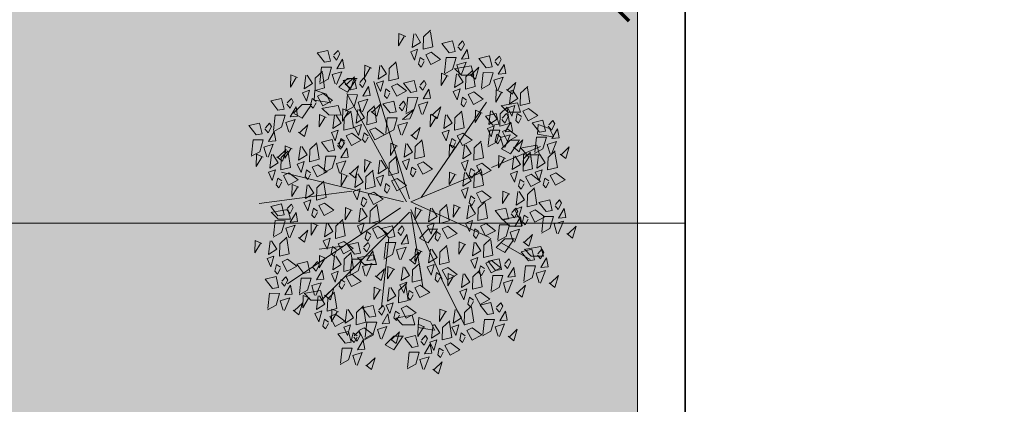
# Model space of a CAD drawing. Units: inches. Extents: x 1704 to 6393, y -157 to 1172.
# Tile 92 of 122: x 2667 to 2750, y 880 to 912. Entities that reach past the tile are written whole.
import ezdxf

# ---------------------------------------------------------------- set-up
doc = ezdxf.new("R2010")
doc.units = ezdxf.units.IN
doc.header["$MEASUREMENT"] = 0
for name, color, linetype, lineweight in [('A-ANNO-DIMS', 7, 'Continuous', 13), ('C-PROP', 7, 'Continuous', 35), ('L-HRDS', 8, 'Continuous', 18), ('L-shrub', 74, 'Continuous', 18)]:
    doc.layers.add(name, color=color, linetype=linetype, lineweight=lineweight)
doc.layers.add('L-HRDS-PATT', color=9, linetype='Continuous', lineweight=13, true_color=0xc5c1ba)
doc.styles.get("Standard").update_dxf_attribs({"font": 'arial.ttf'})
doc.dimstyles.get("Standard").update_dxf_attribs({"dimtxt": 6, "dimasz": 2, "dimexe": 0.18, "dimexo": 0.0625, "dimgap": 0.09, "dimtad": 0, "dimtih": 1, "dimtoh": 1, "dimdec": 1, "dimzin": 0, "dimdsep": 46, "dimlunit": 3, "dimtxsty": 'Standard', "dimblk": 'ARCHTICK', "dimcen": 0.09, "dimadec": 0, "dimazin": 0, "dimtfac": 1, "dimtdec": 1, "dimtofl": 0, "dimtmove": 0, "dimatfit": 3, "dimfxl": 1, "dimtolj": 1, "dimtzin": 0, "dimarcsym": 0})

# ---------------------------------------------------------------- blocks, each defined once
blk = doc.blocks.new('flower shrub 3')
at = {"layer": 'L-shrub'}
for p, q in [((-130.4, 216.9), (-123.5, 236)), ((-123.5, 236), (-109, 242.8)), ((-109.8, 240.6), (-114, 215.7)), ((-114, 215.7), (-130.4, 216.9)), ((-96, 214.8), (-80.2, 219.2)), ((-91.6, 189.9), (-96, 214.8)), ((-80.2, 219.2), (-80.3, 198.9)), ((71.1, 221.6), (86.9, 226)), ((75.6, 196.7), (71.1, 221.6)), ((86.9, 226), (86.9, 205.7)), ((-80.3, 198.9), (-91.6, 187.7)), ((86.9, 205.7), (75.5, 194.4)), ((-166.1, 183.2), (-150.2, 187.7)), ((-161.6, 158.3), (-166.1, 183.2)), ((-150.2, 187.7), (-150.3, 167.3)), ((-104.3, 171), (-104.5, 187)), ((-102.9, 185.4), (-82, 171.2)), ((21.4, 185.5), (37.3, 189.9)), ((25.9, 160.6), (21.4, 185.5)), ((37.3, 189.9), (37.2, 169.6)), ((-150.3, 167.3), (-161.6, 156.1)), ((-89.8, 156.8), (-104.3, 171)), ((-82, 171.2), (-89.8, 156.8)), ((37.2, 169.6), (25.8, 158.3)), ((58.3, 162), (58.1, 177.9)), ((59.8, 176.3), (80.7, 162.2)), ((72.8, 147.7), (58.3, 162)), ((80.7, 162.2), (72.8, 147.7)), ((-227, 106.5), (-211.2, 110.9)), ((-222.6, 81.6), (-227, 106.5)), ((-211.2, 110.9), (-211.3, 90.6)), ((-211.3, 90.6), (-222.6, 79.4)), ((42.5, 35.6), (42.3, 51.6)), ((43.9, 50), (64.8, 35.8)), ((57, 21.4), (42.5, 35.6)), ((64.8, 35.8), (57, 21.4)), ((188.1, 20.6), (195.1, 39.7)), ((195.1, 39.7), (209.5, 46.5)), ((208.7, 44.3), (204.5, 19.5)), ((204.5, 19.5), (188.1, 20.6)), ((184.1, 9.5), (199.9, 13.9)), ((188.5, -15.4), (184.1, 9.5)), ((199.9, 13.9), (199.8, -6.4)), ((199.8, -6.4), (188.5, -17.7)), ((218.7, -20.8), (218.5, -4.8)), ((220.1, -6.4), (241, -20.6)), ((233.2, -35), (218.7, -20.8)), ((241, -20.6), (233.2, -35)), ((84.7, -53.7), (100.5, -49.2)), ((89.1, -78.6), (84.7, -53.7)), ((100.5, -49.2), (100.4, -69.6)), ((100.4, -69.6), (89.1, -80.8)), ((-206, -97.5), (-206.1, -81.5)), ((-204.5, -83.1), (-183.6, -97.3)), ((-183.6, -97.3), (-191.5, -111.7)), ((-191.5, -111.7), (-206, -97.5)), ((-161.5, -112.4), (-145.7, -107.9)), ((-157.1, -137.2), (-161.5, -112.4)), ((-145.7, -107.9), (-145.8, -128.2)), ((-179.9, -131.8), (-165.5, -125)), ((-166.2, -127.1), (-170.5, -152)), ((-145.8, -128.2), (-157.1, -139.5)), ((-186.9, -150.9), (-179.9, -131.8)), ((143.4, -141.7), (159.2, -137.2)), ((147.8, -166.6), (143.4, -141.7)), ((159.2, -137.2), (159.2, -157.6)), ((-170.5, -152), (-186.9, -150.9)), ((-163.1, -171.9), (-163.2, -156)), ((-161.6, -157.6), (-140.7, -171.7)), ((159.2, -157.6), (147.8, -168.8)), ((-148.6, -186.2), (-163.1, -171.9)), ((-140.7, -171.7), (-148.6, -186.2)), ((10.1, -195.8), (26, -191.4)), ((26, -191.4), (25.9, -211.7)), ((14.6, -220.7), (10.1, -195.8)), ((25.9, -211.7), (14.5, -223))]:
    blk.add_line(p, q, dxfattribs=at)
for points in [[(49.5, 264.4), (57, 273.9), (37.6, 279.7), (50.2, 266.6)], [(-81.5, 253.1), (-74, 262.7), (-93.5, 268.4), (-80.9, 255.3)], [(-50.4, 246.2), (-38.7, 261.6), (-30.1, 245.6), (-46.1, 237), (-50.4, 246.2)], [(24.3, 250.7), (23.1, 262.8), (8.2, 260.2), (24.3, 250.7)], [(-127.3, 233.7), (-121, 238.9), (-131.2, 244.3), (-136.8, 241.3), (-129.5, 234.4)], [(-106.8, 239.4), (-107.9, 251.5), (-122.8, 248.9), (-106.8, 239.4)], [(-81.7, 236.7), (-97.2, 231.9), (-102, 247.4), (-81, 238.9)], [(-84.3, 244.8), (-59.4, 248.7), (-55.3, 232.7), (-75.6, 233.3), (-86.6, 244.9)], [(3.7, 245), (10, 250.2), (-0.2, 255.6), (-5.8, 252.5), (1.6, 245.7)], [(49.4, 248), (33.8, 243.2), (29, 258.7), (50, 250.1)], [(130.8, 235.1), (138.4, 244.6), (118.9, 250.4), (131.5, 237.2)], [(-117.5, 219.1), (-132.8, 207.1), (-137, 224.8), (-119.3, 229), (-117.5, 219.1)], [(-84.4, 211.6), (-109.5, 214.3), (-109.3, 230.8), (-89.8, 225), (-82.2, 211)], [(-80.5, 219.9), (-66.7, 228.5), (-58, 214.8), (-80.5, 217.6)], [(-37.1, 234.5), (-41.8, 227.9), (-30.6, 225.3), (-26, 229.7), (-34.9, 234.5)], [(13.5, 230.4), (-1.8, 218.4), (-6, 236.1), (11.8, 240.3), (13.5, 230.4)], [(10.6, 212.3), (22.3, 227.8), (30.9, 211.8), (14.9, 203.2), (10.6, 212.3)], [(46.7, 222.9), (21.5, 225.6), (21.7, 242.1), (41.2, 236.3), (48.8, 222.3)], [(105.6, 221.4), (104.4, 233.5), (89.5, 230.8), (105.6, 221.4)], [(130.7, 218.7), (115.1, 213.8), (110.3, 229.4), (131.3, 220.8)], [(-156.6, 201), (-144.8, 216.5), (-136.2, 200.5), (-152.3, 191.9), (-156.6, 201)], [(-59.4, 140), (-93.7, 220.8)], [(-55.5, 223.7), (-51.3, 212.3), (-37.6, 218.7), (-55.5, 223.7)], [(-48.1, 205.5), (-36.4, 221), (-27.8, 205), (-43.9, 196.4), (-48.1, 205.5)], [(-23.3, 211), (1.6, 214.8), (5.7, 198.9), (-14.6, 199.5), (-25.6, 211)], [(85, 215.7), (91.3, 220.9), (81.1, 226.3), (75.5, 223.2), (82.9, 216.3)], [(128, 193.6), (102.9, 196.3), (103, 212.7), (122.5, 207), (130.1, 192.9)], [(-190.5, 199.7), (-165.5, 203.5), (-161.4, 187.6), (-181.8, 188.2), (-192.7, 199.8)], [(-82.1, 204.2), (-57.1, 208), (-53, 192.1), (-73.3, 192.7), (-84.3, 204.3)], [(-76.4, 204), (-81.2, 192.8), (-60.9, 192.3), (-76.4, 201.7)], [(23.9, 200.7), (19.2, 194), (30.4, 191.5), (35, 195.9), (26.1, 200.6)], [(63.1, 192.2), (70.6, 201.7), (51.1, 207.5), (63.7, 194.4)], [(65.7, 157.2), (92.6, 203.7)], [(94.8, 201), (79.5, 189.1), (75.4, 206.8), (93.1, 211), (94.8, 201)], [(146.6, 180.9), (154.2, 190.5), (134.7, 196.2), (147.3, 183.1)], [(-187.7, 165.1), (-180.1, 174.7), (-199.6, 180.4), (-187, 167.3)], [(-186.6, 174.8), (-172.8, 183.4), (-164.2, 169.6), (-186.7, 172.5)], [(-161.7, 178.6), (-157.5, 167.2), (-143.7, 173.6), (-161.7, 178.6)], [(-143.3, 189.4), (-148, 182.7), (-136.8, 180.2), (-132.1, 184.6), (-141, 189.3)], [(-122.7, 167.2), (-111, 182.7), (-102.3, 166.6), (-118.4, 158), (-122.7, 167.2)], [(-92.8, 176.4), (-85.3, 186), (-104.8, 191.7), (-92.2, 178.6)], [(-78.2, 179.3), (-64.4, 187.9), (-55.7, 174.2), (-78.3, 177)], [(-53.2, 183.1), (-49, 171.7), (-35.3, 178.1), (-53.2, 183.1)], [(-34.9, 193.9), (-39.6, 187.3), (-28.3, 184.7), (-23.7, 189.1), (-32.6, 193.8)], [(-19.5, 186), (-5.7, 194.7), (3, 180.9), (-19.5, 183.8)], [(5.5, 189.9), (9.7, 178.5), (23.4, 184.9), (5.5, 189.9)], [(17.3, 172.8), (23.5, 178), (13.3, 183.4), (7.7, 180.4), (15.1, 173.5)], [(37.8, 178.5), (36.7, 190.6), (21.8, 188), (37.8, 178.5)], [(62.9, 175.8), (47.4, 171), (42.5, 186.5), (63.6, 177.9)], [(121.4, 167.2), (120.3, 179.3), (105.3, 176.7), (121.4, 167.2)], [(218.9, 167.4), (226.5, 176.9), (207, 182.7), (219.6, 169.6)], [(-212.9, 151.4), (-214.1, 163.5), (-229, 160.9), (-212.9, 151.4)], [(-156.6, 165.8), (-131.6, 169.7), (-127.5, 153.8), (-147.9, 154.3), (-158.9, 165.9)], [(-138.6, 157), (-132.3, 162.2), (-142.5, 167.6), (-148.1, 164.6), (-140.8, 157.7)], [(-118.1, 162.7), (-119.2, 174.8), (-134.1, 172.2), (-118.1, 162.7)], [(-92.9, 160), (-108.5, 155.2), (-113.3, 170.7), (-92.3, 162.2)], [(-74.1, 163.4), (-78.9, 152.2), (-58.6, 151.7), (-74.2, 161.1)], [(-15.4, 170.1), (-20.2, 159), (0.1, 158.4), (-15.4, 167.9)], [(27.1, 158.2), (11.8, 146.2), (7.6, 163.9), (25.3, 168.1), (27.1, 158.2)], [(60.2, 150.7), (35.1, 153.4), (35.3, 169.9), (54.7, 164.1), (62.4, 150.1)], [(100.9, 161.5), (107.1, 166.7), (96.9, 172.1), (91.3, 169.1), (98.7, 162.2)], [(146.5, 164.5), (130.9, 159.7), (126.1, 175.2), (147.1, 166.7)], [(193.7, 153.7), (192.5, 165.8), (177.6, 163.1), (193.7, 153.7)], [(-233.5, 145.7), (-227.2, 151), (-237.4, 156.3), (-243, 153.3), (-235.6, 146.4)], [(-187.8, 148.7), (-203.4, 143.9), (-208.2, 159.4), (-187.2, 150.9)], [(-182.5, 158.9), (-187.4, 147.7), (-167, 147.1), (-182.6, 156.6)], [(-152.8, 140.9), (-139, 149.6), (-130.3, 135.8), (-152.8, 138.7)], [(-128.8, 142.4), (-144.1, 130.4), (-148.3, 148.1), (-130.6, 152.3), (-128.8, 142.4)], [(-95.7, 134.9), (-120.8, 137.6), (-120.6, 154.1), (-101.1, 148.3), (-93.5, 134.3)], [(-109.4, 155.5), (-114.1, 148.9), (-102.9, 146.3), (-98.3, 150.7), (-107.2, 155.5)], [(33.2, 131.1), (44.9, 146.6), (53.5, 130.5), (37.5, 121.9), (33.2, 131.1)], [(110.7, 146.9), (95.3, 134.9), (91.2, 152.6), (108.9, 156.8), (110.7, 146.9)], [(94.2, 140.1), (105.9, 155.6), (114.5, 139.6), (98.5, 131), (94.2, 140.1)], [(143.8, 139.4), (118.7, 142.1), (118.8, 158.6), (138.3, 152.8), (146, 138.8)], [(173.1, 148), (179.4, 153.2), (169.2, 158.6), (163.6, 155.5), (171, 148.6)], [(218.8, 151), (203.2, 146.2), (198.4, 161.7), (219.4, 153.1)], [(-223.7, 131.1), (-239, 119.1), (-243.2, 136.9), (-225.4, 141), (-223.7, 131.1)], [(-190.5, 123.6), (-215.6, 126.4), (-215.5, 142.8), (-196, 137), (-188.4, 123)], [(-9.9, 24.3), (-166.8, 132)], [(-127.8, 144.8), (-123.6, 133.4), (-109.9, 139.8), (-127.8, 144.8)], [(-66.2, 124.3), (-54.5, 139.8), (-45.9, 123.8), (-61.9, 115.2), (-66.2, 124.3)], [(-21, 124.3), (-9.3, 139.8), (-0.7, 123.8), (-16.7, 115.2), (-21, 124.3)], [(-0.7, 129.8), (24.2, 133.6), (28.3, 117.7), (8, 118.2), (-3, 129.8)], [(-2.5, 7.1), (56.3, 136.9)], [(60.3, 138.8), (85.2, 142.6), (89.3, 126.7), (69, 127.3), (58, 138.8)], [(146.1, 122.1), (157.9, 137.6), (166.5, 121.5), (150.4, 112.9), (146.1, 122.1)], [(182.9, 133.3), (167.6, 121.4), (163.4, 139.1), (181.2, 143.3), (182.9, 133.3)], [(216.1, 125.9), (191, 128.6), (191.1, 145), (210.6, 139.3), (218.2, 125.2)], [(-212.5, 104.2), (-205, 113.8), (-224.5, 119.5), (-211.9, 106.4)], [(-183.7, 110.8), (-171.9, 126.3), (-163.3, 110.2), (-179.4, 101.6), (-183.7, 110.8)], [(-148.7, 125), (-153.5, 113.9), (-133.2, 113.3), (-148.7, 122.8)], [(-100.1, 123), (-75.2, 126.8), (-71.1, 110.9), (-91.4, 111.5), (-102.4, 123)], [(-54.9, 123), (-30, 126.8), (-25.9, 110.9), (-46.2, 111.5), (-57.2, 123)], [(-2.5, 7.1), (-51.6, 124.7)], [(46.4, 119.4), (41.7, 112.8), (53, 110.2), (57.6, 114.6), (48.7, 119.4)], [(64.1, 113.8), (77.9, 122.5), (86.6, 108.7), (64, 111.6)], [(89.1, 117.7), (93.3, 106.3), (107, 112.7), (89.1, 117.7)], [(107.4, 128.5), (102.7, 121.8), (114, 119.3), (118.6, 123.7), (109.7, 128.4)], [(112.2, 120.7), (137.2, 124.6), (141.3, 108.7), (120.9, 109.2), (110, 120.8)], [(204.9, 108.5), (216.6, 124), (225.2, 108), (209.2, 99.4), (204.9, 108.5)], [(-237.8, 90.5), (-238.9, 102.6), (-253.8, 100), (-237.8, 90.5)], [(-212.7, 87.8), (-228.2, 83), (-233.1, 98.5), (-212, 90)], [(-217.6, 109.4), (-192.6, 113.3), (-188.5, 97.4), (-208.9, 97.9), (-219.9, 109.5)], [(-170.4, 99.1), (-175.1, 92.5), (-163.9, 89.9), (-159.2, 94.3), (-168.2, 99.1)], [(-115.9, 92.7), (-104.2, 108.2), (-95.6, 92.2), (-111.6, 83.6), (-115.9, 92.7)], [(-96.3, 98.1), (-82.5, 106.7), (-73.8, 92.9), (-96.3, 95.8)], [(-71.3, 101.9), (-67.1, 90.5), (-53.4, 96.9), (-71.3, 101.9)], [(-53, 112.7), (-57.6, 106), (-46.4, 103.5), (-41.8, 107.9), (-50.7, 112.6)], [(-51.1, 98.1), (-37.3, 106.7), (-28.6, 92.9), (-51.2, 95.8)], [(-26.1, 101.9), (-21.9, 90.5), (-8.2, 96.9), (-26.1, 101.9)], [(-7.8, 112.7), (-12.5, 106), (-1.2, 103.5), (3.4, 107.9), (-5.5, 112.6)], [(3.1, 104.8), (16.9, 113.5), (25.6, 99.7), (3.1, 102.6)], [(28.1, 108.7), (32.3, 97.3), (46, 103.7), (28.1, 108.7)], [(68.2, 97.9), (63.4, 86.8), (83.7, 86.2), (68.1, 95.7)], [(116.1, 95.8), (129.9, 104.5), (138.5, 90.7), (116, 93.5)], [(141, 99.6), (145.2, 88.2), (159, 94.6), (141, 99.6)], [(159.4, 110.4), (154.7, 103.8), (165.9, 101.2), (170.6, 105.6), (161.6, 110.4)], [(170.9, 107.2), (195.9, 111), (200, 95.1), (179.7, 95.7), (168.7, 107.3)], [(-258.3, 84.8), (-252.1, 90), (-262.2, 95.4), (-267.9, 92.4), (-260.5, 85.5)], [(-215.4, 62.7), (-240.5, 65.4), (-240.3, 81.9), (-220.8, 76.1), (-213.2, 62.1)], [(-213.7, 84.5), (-200, 93.2), (-191.3, 79.4), (-213.8, 82.3)], [(-188.8, 88.4), (-184.6, 77), (-170.8, 83.4), (-188.8, 88.4)], [(-149.8, 91.4), (-124.9, 95.2), (-120.8, 79.3), (-141.1, 79.9), (-152.1, 91.5)], [(-92.2, 82.1), (-97, 71), (-76.7, 70.4), (-92.3, 79.9)], [(-47, 82.1), (-51.8, 71), (-31.5, 70.4), (-47.1, 79.9)], [(7.2, 88.9), (2.4, 77.8), (22.7, 77.2), (7.1, 86.7)], [(37.7, 67.9), (49.4, 83.4), (58, 67.4), (42, 58.8), (37.7, 67.9)], [(105.5, 67.9), (117.2, 83.4), (125.8, 67.4), (109.8, 58.8), (105.5, 67.9)], [(122.1, 56.8), (200.5, 95.9)], [(174.8, 82.3), (188.6, 90.9), (197.3, 77.1), (174.7, 80)], [(199.8, 86.1), (204, 74.7), (217.7, 81.1), (199.8, 86.1)], [(218.1, 96.9), (213.4, 90.2), (224.7, 87.7), (229.3, 92.1), (220.4, 96.8)], [(229.7, 72.4), (241.4, 87.9), (250.1, 71.9), (234, 63.3), (229.7, 72.4)], [(-248.5, 70.2), (-263.8, 58.2), (-268, 75.9), (-250.3, 80.1), (-248.5, 70.2)], [(-209.7, 68.6), (-214.5, 57.5), (-194.2, 56.9), (-209.7, 66.3)], [(-146, 66.5), (-132.2, 75.1), (-123.5, 61.3), (-146, 64.2)], [(-121, 70.3), (-116.8, 58.9), (-103.1, 65.3), (-121, 70.3)], [(-102.6, 81.1), (-107.3, 74.5), (-96.1, 71.9), (-91.5, 76.3), (-100.4, 81)], [(3.8, 66.6), (28.7, 70.4), (32.8, 54.5), (12.5, 55.1), (1.5, 66.6)], [(71.6, 66.6), (96.5, 70.4), (100.6, 54.5), (80.3, 55.1), (69.3, 66.6)], [(120.2, 79.9), (115.3, 68.7), (135.7, 68.2), (120.1, 77.6)], [(178.9, 66.3), (174.1, 55.2), (194.4, 54.6), (178.8, 64.1)], [(195.8, 71.1), (220.8, 74.9), (224.8, 59), (204.5, 59.6), (193.5, 71.2)], [(-249.2, 40.8), (-237.5, 56.3), (-228.8, 40.3), (-244.9, 31.7), (-249.2, 40.8)], [(-147, 41), (-139.5, 50.6), (-159, 56.4), (-146.4, 43.2)], [(-141.9, 50.6), (-146.7, 39.4), (-126.4, 38.9), (-141.9, 48.3)], [(7.6, 41.6), (21.4, 50.3), (30.1, 36.5), (7.6, 39.4)], [(9.7, 7.1), (125, 58.6)], [(51, 56.3), (46.3, 49.6), (57.5, 47.1), (62.1, 51.5), (53.2, 56.2)], [(75.4, 41.6), (89.2, 50.3), (97.9, 36.5), (75.3, 39.4)], [(118.7, 56.3), (114, 49.6), (125.3, 47.1), (129.9, 51.5), (121, 56.2)], [(199.6, 46.2), (213.4, 54.8), (222.1, 41), (199.6, 43.9)], [(224.6, 50), (228.8, 38.6), (242.5, 45), (224.6, 50)], [(243, 60.8), (238.3, 54.1), (249.5, 51.6), (254.1, 56), (245.2, 60.7)], [(273.1, 43.3), (280.7, 52.8), (261.2, 58.6), (273.8, 45.5)], [(-283.1, 39.5), (-258.1, 43.3), (-254.1, 27.4), (-274.4, 28), (-285.4, 39.6)], [(-172.3, 27.3), (-173.4, 39.4), (-188.3, 36.8), (-172.3, 27.3)], [(-147.2, 24.6), (-162.7, 19.8), (-167.5, 35.4), (-146.5, 26.8)], [(-68.5, 27.3), (-56.7, 42.8), (-48.1, 26.8), (-64.2, 18.2), (-68.5, 27.3)], [(32.6, 45.5), (36.8, 34.1), (50.5, 40.5), (32.6, 45.5)], [(100.4, 45.5), (104.6, 34.1), (118.3, 40.5), (100.4, 45.5)], [(134.9, 22.8), (146.6, 38.3), (155.2, 22.2), (139.1, 13.7), (134.9, 22.8)], [(227.4, 23.9), (233.6, 29.1), (223.4, 34.5), (217.8, 31.4), (225.2, 24.6)], [(247.9, 29.6), (246.8, 41.7), (231.8, 39.1), (247.9, 29.6)], [(273, 26.9), (257.4, 22.1), (252.6, 37.6), (273.6, 29)], [(-279.3, 14.6), (-265.5, 23.2), (-256.8, 9.5), (-279.3, 12.3)], [(-254.3, 18.4), (-250.1, 7), (-236.4, 13.4), (-254.3, 18.4)], [(-235.9, 29.2), (-240.6, 22.6), (-229.4, 20), (-224.8, 24.4), (-233.7, 29.1)], [(-183, 7), (-198.3, -4.9), (-202.5, 12.8), (-184.8, 16.9), (-183, 7)], [(-192.8, 21.7), (-186.5, 26.9), (-196.7, 32.2), (-202.4, 29.2), (-195, 22.3)], [(-149.9, -0.5), (-175, 2.3), (-174.8, 18.7), (-155.3, 12.9), (-147.7, -1.1)], [(-113.1, 7.2), (-105.6, 16.7), (-125.1, 22.5), (-112.5, 9.4)], [(-102.4, 26), (-77.4, 29.8), (-73.3, 13.9), (-93.7, 14.4), (-104.6, 26)], [(11.7, 25.7), (6.9, 14.6), (27.2, 14), (11.7, 23.5)], [(14.6, 7.1), (137.2, 26.7)], [(79.5, 25.7), (74.7, 14.6), (95, 14), (79.4, 23.5)], [(92.4, 4.9), (100, 14.5), (80.5, 20.3), (93.1, 7.1)], [(100.9, 21.5), (125.9, 25.3), (130, 9.4), (109.6, 9.9), (98.7, 21.5)], [(203.7, 30.3), (198.9, 19.1), (219.2, 18.5), (203.7, 28)], [(237.2, 9.2), (221.8, -2.7), (217.7, 15), (235.4, 19.2), (237.2, 9.2)], [(270.3, 1.8), (245.2, 4.5), (245.3, 20.9), (264.8, 15.2), (272.5, 1.2)], [(-7.4, 4.7), (-201.1, -54.1)], [(-138.4, -6.5), (-139.5, 5.6), (-154.3, 11.9), (-138.4, -6.5)], [(-113.3, -9.2), (-128.8, -14), (-133.7, 1.5), (-112.6, -7.1)], [(-98.5, 1), (-84.7, 9.7), (-76.1, -4.1), (-98.6, -1.2)], [(-73.6, 4.9), (-69.4, -6.5), (-55.6, -0.1), (-73.6, 4.9)], [(-55.2, 15.7), (-59.9, 9), (-48.7, 6.5), (-44, 10.9), (-53, 15.6)], [(14.6, 4.7), (156.8, -137.4)], [(67.2, -8.8), (66, 3.3), (51.1, 0.7), (67.2, -8.8)], [(104.8, -3.5), (118.6, 5.2), (127.2, -8.6), (104.7, -5.7)], [(129.7, 0.4), (133.9, -11), (147.7, -4.6), (129.7, 0.4)], [(134.8, -1.1), (159.8, 2.7), (163.9, -13.2), (143.5, -12.6), (132.5, -1)], [(148.1, 11.2), (143.4, 4.5), (154.6, 2), (159.3, 6.3), (150.4, 11.1)], [(168.7, 0.2), (180.5, 15.7), (189.1, -0.3), (173, -8.9), (168.7, 0.2)], [(-275.2, -1.3), (-280, -12.5), (-259.7, -13), (-275.2, -3.6)], [(-231.1, -16.9), (-206.2, -13.1), (-202.1, -29), (-222.4, -28.4), (-233.4, -16.8)], [(-197.2, -15.6), (-185.5, -0.1), (-176.9, -16.1), (-192.9, -24.7), (-197.2, -15.6)], [(-2.5, -0.2), (-181.5, -98.2)], [(-158.9, -12.2), (-152.7, -7), (-162.9, -1.6), (-168.5, -4.7), (-161.1, -11.5)], [(-116, -34.3), (-141.1, -31.6), (-140.9, -15.2), (-121.5, -20.9), (-113.8, -34.9)], [(-94.4, -14.9), (-99.3, -26), (-78.9, -26.6), (-94.5, -17.1)], [(-75.3, -16.9), (-50.3, -13.1), (-46.2, -29), (-66.6, -28.4), (-77.5, -16.8)], [(-2.5, -5.1), (-51.6, -205.9)], [(-41.3, -15.6), (-29.6, -0.1), (-21, -16.1), (-37.1, -24.7), (-41.3, -15.6)], [(7.3, -10), (132.3, -196.1)], [(46.6, -14.4), (52.9, -9.2), (42.7, -3.9), (37.1, -6.9), (44.5, -13.8)], [(92.3, -11.5), (76.7, -16.3), (71.9, -0.7), (92.9, -9.3)], [(182, -11.4), (177.3, -18.1), (188.5, -20.6), (193.1, -16.2), (184.2, -11.5)], [(223.5, -26.6), (231, -17.1), (211.5, -11.3), (224.1, -24.5)], [(-184, -27.2), (-188.7, -33.8), (-177.4, -36.4), (-172.8, -32), (-181.7, -27.3)], [(-149.1, -26.8), (-164.4, -38.8), (-168.6, -21.1), (-150.9, -16.9), (-149.1, -26.8)], [(-28.1, -27.2), (-32.8, -33.8), (-21.6, -36.4), (-16.9, -32), (-25.8, -27.3)], [(56.4, -29.1), (41.1, -41), (36.9, -23.3), (54.7, -19.2), (56.4, -29.1)], [(37.7, -47.1), (49.4, -31.7), (58, -47.7), (42, -56.3), (37.7, -47.1)], [(55.9, -29), (171.1, -41.2)], [(89.6, -36.6), (64.5, -33.8), (64.6, -17.4), (84.1, -23.2), (91.7, -37.2)], [(108.9, -19.4), (104, -30.5), (124.4, -31.1), (108.8, -21.6)], [(138.6, -26), (152.4, -17.4), (161.1, -31.2), (138.6, -28.3)], [(163.6, -22.2), (167.8, -33.6), (181.6, -27.2), (163.6, -22.2)], [(198.2, -40.3), (197.1, -28.2), (182.1, -30.9), (198.2, -40.3)], [(223.3, -43.1), (207.7, -47.9), (202.9, -32.3), (223.9, -40.9)], [(-227.3, -41.8), (-213.5, -33.2), (-204.8, -46.9), (-227.4, -44.1)], [(-202.3, -38), (-198.1, -49.4), (-184.4, -43), (-202.3, -38)], [(-151.5, -58.2), (-144, -48.7), (-163.5, -42.9), (-150.9, -56.1)], [(-124.9, -51.7), (-113.2, -36.2), (-104.6, -52.2), (-120.7, -60.8), (-124.9, -51.7)], [(-71.4, -41.8), (-57.6, -33.2), (-49, -46.9), (-71.5, -44.1)], [(-46.5, -38), (-42.3, -49.4), (-28.5, -43), (-46.5, -38)], [(-18.8, -53.9), (-7, -38.4), (1.6, -54.5), (-14.5, -63.1), (-18.8, -53.9)], [(3.8, -48.5), (28.7, -44.6), (32.8, -60.6), (12.5, -60), (1.5, -48.4)], [(119.5, -51.5), (127.1, -41.9), (107.6, -36.2), (120.2, -49.3)], [(142.7, -41.9), (137.9, -53.1), (158.2, -53.6), (142.7, -44.2)], [(177.7, -46), (183.9, -40.8), (173.7, -35.5), (168.1, -38.5), (175.5, -45.4)], [(-223.2, -57.7), (-228, -68.9), (-207.7, -69.4), (-223.3, -60)], [(-176.8, -71.9), (-177.9, -59.8), (-192.8, -62.5), (-176.8, -71.9)], [(-151.7, -74.6), (-167.2, -79.5), (-172.1, -63.9), (-151, -72.5)], [(-158.9, -53), (-133.9, -49.2), (-129.8, -65.1), (-150.1, -64.5), (-161.1, -52.9)], [(-111.7, -63.3), (-116.4, -69.9), (-105.2, -72.5), (-100.5, -68.1), (-109.4, -63.4)], [(-67.3, -57.7), (-72.2, -68.9), (-51.8, -69.4), (-67.4, -60)], [(-52.7, -55.3), (-27.7, -51.4), (-23.6, -67.3), (-44, -66.8), (-54.9, -55.2)], [(7.6, -73.4), (21.4, -64.8), (30.1, -78.5), (7.6, -75.7)], [(51, -58.8), (46.3, -65.4), (57.5, -68), (62.1, -63.6), (53.2, -58.8)], [(73.8, -70.8), (80, -65.6), (69.8, -60.3), (64.2, -63.3), (71.6, -70.2)], [(94.3, -65.2), (93.2, -53.1), (78.2, -55.7), (94.3, -65.2)], [(119.4, -67.9), (103.8, -72.7), (99, -57.1), (120, -65.7)], [(187.5, -60.7), (172.1, -72.6), (168, -54.9), (185.7, -50.8), (187.5, -60.7)], [(220.6, -68.1), (195.5, -65.4), (195.6, -49), (215.1, -54.8), (222.8, -68.8)], [(204.9, -69.7), (216.6, -54.2), (225.2, -70.3), (209.2, -78.8), (204.9, -69.7)], [(266.4, -67.2), (273.9, -57.7), (254.4, -51.9), (267, -65.1)], [(-197.3, -77.6), (-191.1, -72.4), (-201.3, -67), (-206.9, -70.1), (-199.5, -77)], [(-154.4, -99.7), (-179.5, -97), (-179.3, -80.6), (-159.9, -86.3), (-152.2, -100.4)], [(-155, -77.9), (-141.2, -69.3), (-132.6, -83), (-155.1, -80.2)], [(-130.1, -74.1), (-125.8, -85.5), (-112.1, -79.1), (-130.1, -74.1)], [(-115.9, -90), (-104.2, -74.5), (-95.6, -90.6), (-111.6, -99.2), (-115.9, -90)], [(-49.9, -94.3), (-42.3, -84.8), (-61.8, -79), (-49.2, -92.2)], [(-48.8, -80.2), (-35.1, -71.5), (-26.4, -85.3), (-48.9, -82.4)], [(-23.9, -76.3), (-19.7, -87.7), (-5.9, -81.3), (-23.9, -76.3)], [(-5.5, -65.6), (-10.2, -72.2), (1, -74.8), (5.7, -70.4), (-3.3, -65.6)], [(32.6, -69.6), (36.8, -81), (50.5, -74.6), (32.6, -69.6)], [(83.6, -85.5), (68.2, -97.4), (64.1, -79.7), (81.8, -75.6), (83.6, -85.5)], [(116.7, -93), (91.6, -90.2), (91.7, -73.8), (111.2, -79.6), (118.8, -93.6)], [(116.8, -90), (128.5, -74.5), (137.1, -90.6), (121.1, -99.2), (116.8, -90)], [(170.9, -71), (195.9, -67.2), (200, -83.1), (179.7, -82.6), (168.7, -71)], [(220.6, -86.6), (226.8, -81.4), (216.6, -76.1), (211, -79.1), (218.4, -86)], [(241.1, -80.9), (240, -68.9), (225.1, -71.5), (241.1, -80.9)], [(266.2, -83.7), (250.7, -88.5), (245.8, -72.9), (266.9, -81.5)], [(-196.7, -101.1), (-189.2, -91.6), (-208.7, -85.8), (-196.1, -98.9)], [(-187.5, -92.3), (-202.8, -104.2), (-207, -86.5), (-189.3, -82.3), (-187.5, -92.3)], [(-150.9, -93.8), (-155.7, -105), (-135.4, -105.5), (-151, -96.1)], [(-149.8, -91.4), (-124.9, -87.5), (-120.8, -103.4), (-141.1, -102.9), (-152.1, -91.3)], [(-75.1, -108), (-76.3, -95.9), (-91.2, -98.6), (-75.1, -108)], [(-44.8, -96.1), (-49.6, -107.2), (-29.3, -107.8), (-44.8, -98.3)], [(-12.8, -149), (-20.2, -90.2)], [(11.7, -89.3), (6.9, -100.5), (27.2, -101), (11.7, -91.6)], [(62.6, -103.5), (74.3, -88.1), (82.9, -104.1), (66.8, -112.7), (62.6, -103.5)], [(82.8, -91.4), (107.8, -87.5), (111.9, -103.4), (91.6, -102.9), (80.6, -91.3)], [(174.8, -96), (188.6, -87.3), (197.3, -101.1), (174.7, -98.2)], [(199.8, -92.1), (204, -103.5), (217.7, -97.1), (199.8, -92.1)], [(230.4, -101.3), (215.1, -113.2), (210.9, -95.5), (228.6, -91.4), (230.4, -101.3)], [(218.1, -81.3), (213.4, -88), (224.7, -90.6), (229.3, -86.2), (220.4, -81.4)], [(263.5, -108.8), (238.4, -106), (238.6, -89.6), (258, -95.4), (265.7, -109.4)], [(-242.5, -120.5), (-236.2, -115.3), (-246.4, -109.9), (-252, -112.9), (-244.7, -119.8)], [(-222, -114.8), (-223.1, -102.7), (-238, -105.3), (-222, -114.8)], [(-196.9, -117.5), (-212.4, -122.3), (-217.2, -106.8), (-196.2, -115.4)], [(-146, -116.3), (-132.2, -107.6), (-123.5, -121.4), (-146, -118.5)], [(-121, -112.4), (-116.8, -123.8), (-103.1, -117.4), (-121, -112.4)], [(-102.6, -101.7), (-107.3, -108.3), (-96.1, -110.9), (-91.5, -106.5), (-100.4, -101.7)], [(-95.7, -113.7), (-89.4, -108.5), (-99.6, -103.1), (-105.2, -106.2), (-97.8, -113.1)], [(-50, -110.7), (-65.6, -115.6), (-70.4, -100), (-49.4, -108.6)], [(28.6, -104.9), (53.6, -101), (57.7, -117), (37.4, -116.4), (26.4, -104.8)], [(70.6, -104.9), (75.5, -144.1)], [(86.7, -116.3), (100.5, -107.6), (109.2, -121.4), (86.6, -118.5)], [(111.7, -112.4), (115.9, -123.8), (129.6, -117.4), (111.7, -112.4)], [(130, -101.7), (125.3, -108.3), (136.6, -110.9), (141.2, -106.5), (132.3, -101.7)], [(178.9, -111.9), (174.1, -123), (194.4, -123.6), (178.8, -114.1)], [(182.3, -117.1), (194, -101.6), (202.6, -117.6), (186.6, -126.2), (182.3, -117.1)], [(-232.7, -135.1), (-248, -147.1), (-252.2, -129.4), (-234.5, -125.2), (-232.7, -135.1)], [(-199.6, -142.6), (-224.7, -139.9), (-224.5, -123.4), (-205, -129.2), (-197.4, -143.2)], [(-181.4, -137.4), (-169.7, -121.9), (-161.1, -137.9), (-177.1, -146.5), (-181.4, -137.4)], [(-85.9, -128.4), (-101.2, -140.3), (-105.4, -122.6), (-87.6, -118.4), (-85.9, -128.4)], [(-52.7, -135.8), (-77.8, -133.1), (-77.7, -116.7), (-58.2, -122.4), (-50.6, -136.5)], [(-0.7, -135.1), (11, -119.7), (19.6, -135.7), (3.6, -144.3), (-0.7, -135.1)], [(32.5, -129.8), (46.3, -121.2), (54.9, -134.9), (32.4, -132.1)], [(57.4, -126), (61.7, -137.4), (75.4, -131), (57.4, -126)], [(75.8, -115.2), (71.1, -121.8), (82.3, -124.4), (87, -120), (78.1, -115.3)], [(151.2, -134.9), (158.7, -125.4), (139.2, -119.6), (151.8, -132.8)], [(148.4, -118.4), (173.3, -114.6), (177.4, -130.5), (157.1, -129.9), (146.1, -118.4)], [(195.5, -128.7), (190.8, -135.4), (202.1, -137.9), (206.7, -133.5), (197.8, -128.8)], [(-215.3, -138.7), (-190.4, -134.9), (-186.3, -150.8), (-206.6, -150.3), (-217.6, -138.7)], [(-141.9, -132.2), (-146.7, -143.3), (-126.4, -143.9), (-141.9, -134.4)], [(-97.9, -147.8), (-72.9, -143.9), (-68.8, -159.8), (-89.1, -159.3), (-100.1, -147.7)], [(-63.9, -146.4), (-52.2, -130.9), (-43.6, -147), (-59.7, -155.6), (-63.9, -146.4)], [(-34.6, -136.5), (-9.7, -132.6), (-5.6, -148.5), (-25.9, -148), (-36.9, -136.4)], [(36.6, -145.7), (31.7, -156.9), (52.1, -157.4), (36.5, -148)], [(90.8, -132.2), (86, -143.3), (106.3, -143.9), (90.7, -134.4)], [(105.4, -154.3), (111.6, -149.1), (101.4, -143.7), (95.8, -146.8), (103.2, -153.7)], [(125.9, -148.6), (124.8, -136.5), (109.9, -139.2), (125.9, -148.6)], [(151, -151.4), (135.5, -156.2), (130.6, -140.6), (151.7, -149.2)], [(152.2, -143.4), (166, -134.7), (174.7, -148.5), (152.1, -145.6)], [(177.2, -139.5), (181.4, -150.9), (195.1, -144.5), (177.2, -139.5)], [(-211.5, -163.7), (-197.7, -155), (-189, -168.8), (-211.5, -165.9)], [(-186.5, -159.8), (-182.3, -171.2), (-168.6, -164.8), (-186.5, -159.8)], [(-168.2, -149), (-172.9, -155.7), (-161.6, -158.2), (-157, -153.8), (-165.9, -149.1)], [(-50.7, -158.1), (-55.4, -164.7), (-44.2, -167.3), (-39.5, -162.9), (-48.4, -158.1)], [(-30.8, -161.4), (-17, -152.7), (-8.3, -166.5), (-30.8, -163.7)], [(-12.3, -147.2), (-0.1, -242.7)], [(-5.8, -157.6), (-1.6, -169), (12.1, -162.6), (-5.8, -157.6)], [(12.6, -146.8), (7.9, -153.4), (19.1, -156), (23.7, -151.6), (14.8, -146.8)], [(115.2, -169), (99.9, -180.9), (95.7, -163.2), (113.4, -159.1), (115.2, -169)], [(148.3, -176.4), (123.2, -173.7), (123.3, -157.3), (142.8, -163.1), (150.5, -177.1)], [(156.3, -159.3), (151.5, -170.4), (171.8, -171), (156.2, -161.5)], [(-117.6, -177.8), (-110.1, -168.3), (-129.6, -162.5), (-117, -175.6)], [(-94, -172.7), (-80.2, -164), (-71.6, -177.8), (-94.1, -174.9)], [(-69.1, -168.8), (-64.8, -180.2), (-51.1, -173.8), (-69.1, -168.8)], [(-50.4, -193.8), (-38.7, -178.3), (-30.1, -194.3), (-46.1, -202.9), (-50.4, -193.8)], [(-26.7, -177.3), (-31.5, -188.5), (-11.2, -189), (-26.7, -179.6)], [(56.3, -177.8), (63.8, -168.3), (44.3, -162.5), (56.9, -175.6)], [(176, -186.8), (183.5, -177.3), (164.1, -171.5), (176.7, -184.7)], [(-207.4, -179.6), (-212.2, -190.7), (-191.9, -191.3), (-207.5, -181.8)], [(-163.4, -197.2), (-157.2, -192), (-167.4, -186.6), (-173, -189.7), (-165.6, -196.5)], [(-142.9, -191.5), (-144, -179.4), (-159, -182), (-142.9, -191.5)], [(-117.8, -194.2), (-133.4, -199), (-138.2, -183.5), (-117.2, -192.1)], [(-89.9, -188.6), (-94.8, -199.8), (-74.4, -200.3), (-90, -190.9)], [(-84.3, -195.1), (-59.4, -191.3), (-55.3, -207.2), (-75.6, -206.7), (-86.6, -195.1)], [(10.5, -197.2), (16.8, -192), (6.6, -186.6), (1, -189.7), (8.3, -196.5)], [(31, -191.5), (29.9, -179.4), (15, -182), (31, -191.5)], [(56.1, -194.2), (40.6, -199), (35.8, -183.5), (56.8, -192.1)], [(58, -197.4), (83, -193.6), (87.1, -209.5), (66.7, -208.9), (55.7, -197.3)], [(91.9, -196.1), (103.6, -180.6), (112.3, -196.6), (96.2, -205.2), (91.9, -196.1)], [(150.8, -200.5), (149.6, -188.4), (134.7, -191.1), (150.8, -200.5)], [(175.9, -203.3), (160.3, -208.1), (155.5, -192.5), (176.5, -201.1)], [(-153.6, -211.9), (-169, -223.8), (-173.1, -206.1), (-155.4, -201.9), (-153.6, -211.9)], [(-120.5, -219.3), (-145.6, -216.6), (-145.5, -200.2), (-126, -205.9), (-118.3, -219.9)], [(-77, -213.9), (-69.5, -204.4), (-88.9, -198.6), (-76.3, -211.7)], [(-37.1, -205.4), (-41.8, -212.1), (-30.6, -214.6), (-26, -210.3), (-34.9, -205.5)], [(20.3, -211.9), (5, -223.8), (0.8, -206.1), (18.5, -201.9), (20.3, -211.9)], [(53.4, -219.3), (28.3, -216.6), (28.5, -200.2), (48, -205.9), (55.6, -219.9)], [(105.2, -207.7), (100.5, -214.3), (111.7, -216.9), (116.3, -212.5), (107.4, -207.8)], [(140, -220.9), (124.7, -232.8), (120.5, -215.1), (138.3, -210.9), (140, -220.9)], [(130.2, -206.2), (136.5, -201), (126.3, -195.6), (120.7, -198.7), (128.1, -205.6)], [(173.2, -228.3), (148, -225.6), (148.2, -209.2), (167.7, -214.9), (175.3, -229)], [(-122.8, -233.3), (-116.5, -228.1), (-126.7, -222.7), (-132.3, -225.8), (-124.9, -232.6)], [(-102.2, -227.6), (-103.4, -215.5), (-118.3, -218.1), (-102.2, -227.6)], [(-77.1, -230.3), (-92.7, -235.1), (-97.5, -219.6), (-76.5, -228.2)], [(-80.5, -220.1), (-66.7, -211.4), (-58, -225.2), (-80.5, -222.3)], [(-55.5, -216.2), (-51.3, -227.6), (-37.6, -221.2), (-55.5, -216.2)], [(61.8, -222.3), (75.6, -213.7), (84.3, -227.4), (61.8, -224.6)], [(86.8, -218.5), (91, -229.9), (104.7, -223.5), (86.8, -218.5)], [(-113, -248), (-128.3, -259.9), (-132.5, -242.2), (-114.7, -238), (-113, -248)], [(-79.8, -255.4), (-105, -252.7), (-104.8, -236.3), (-85.3, -242), (-77.7, -256)], [(-76.4, -236), (-81.2, -247.1), (-60.9, -247.7), (-76.4, -238.2)], [(65.9, -238.2), (61.1, -249.4), (81.4, -249.9), (65.9, -240.5)]]:
    blk.add_lwpolyline(points, dxfattribs=at)
blk = doc.blocks.new('_ArchTick')
at = {"color": 0, "linetype": 'ByBlock', "const_width": 0.15}
blk.add_lwpolyline([(-0.5, -0.5), (0.5, 0.5)], dxfattribs=at)
blk = doc.blocks.new('*D84')
at = {"layer": 'A-ANNO-DIMS', "color": 0, "lineweight": -2, "transparency": 16777216}
for p, q in [((2713.724, 939.698), (2717.812, 939.698)), ((2717.632, 939.698), (2717.632, 929.658)), ((2717.632, 913.234), (2717.632, 923.274)), ((2713.724, 913.234), (2717.812, 913.234))]:
    blk.add_line(p, q, dxfattribs=at)
at = {"layer": 'Defpoints', "color": 0, "lineweight": -3, "transparency": 16777216}
for p in [(2713.662, 939.698), (2713.662, 913.234), (2717.632, 913.234)]:
    blk.add_point(p, dxfattribs=at)
at = {"layer": 'A-ANNO-DIMS', "color": 0, "lineweight": -2, "transparency": 16777216, "xscale": 2, "yscale": 2, "zscale": 2}
for p, rotation in [((2717.632, 939.698), 90), ((2717.632, 913.234), 270)]:
    blk.add_blockref('_ArchTick', p, dxfattribs=dict(at, rotation=rotation))
at = {"layer": 'A-ANNO-DIMS', "color": 0, "transparency": 16777216, "insert": (2717.632, 926.466), "char_height": 6, "attachment_point": 5}
blk.add_mtext('\\A1;SHRUB B 26 TYP.', dxfattribs=at)
blk = doc.blocks.new('*D91')
at = {"layer": 'A-ANNO-DIMS', "color": 0, "lineweight": -2, "transparency": 16777216}
for p, q in [((2723.411, 1033.213), (2784.529, 1033.213)), ((2784.349, 1033.213), (2784.349, 517.868)), ((2784.349, -3.787), (2784.349, 511.557)), ((2723.411, -3.787), (2784.529, -3.787))]:
    blk.add_line(p, q, dxfattribs=at)
at = {"layer": 'Defpoints', "color": 0, "lineweight": -3, "transparency": 16777216}
for p in [(2723.349, 1033.213), (2784.349, 1033.213), (2723.349, -3.787)]:
    blk.add_point(p, dxfattribs=at)
at = {"layer": 'A-ANNO-DIMS', "color": 0, "lineweight": -2, "transparency": 16777216, "xscale": 2, "yscale": 2, "zscale": 2}
for p, rotation in [((2784.349, 1033.213), 90), ((2784.349, -3.787), 270)]:
    blk.add_blockref('_ArchTick', p, dxfattribs=dict(at, rotation=rotation))
at = {"layer": 'A-ANNO-DIMS', "color": 0, "transparency": 16777216, "insert": (2784.349, 514.713), "char_height": 6, "attachment_point": 5}
blk.add_mtext('\\A1;1037', dxfattribs=at)
blk = doc.blocks.new('*D95')
at = {"layer": 'A-ANNO-DIMS', "color": 0, "lineweight": -2, "transparency": 16777216}
for p, q in [((2605.349, 895.275), (2605.349, 1105.287)), ((2605.349, 1105.107), (2657.907, 1105.107)), ((2723.349, 1105.107), (2670.791, 1105.107)), ((2723.349, 895.275), (2723.349, 1105.287))]:
    blk.add_line(p, q, dxfattribs=at)
at = {"layer": 'Defpoints', "color": 0, "lineweight": -3, "transparency": 16777216}
for p in [(2723.349, 1105.107), (2605.349, 895.213), (2723.349, 895.213)]:
    blk.add_point(p, dxfattribs=at)
at = {"layer": 'A-ANNO-DIMS', "color": 0, "lineweight": -2, "transparency": 16777216, "xscale": 2, "yscale": 2, "zscale": 2, "rotation": 180}
blk.add_blockref('_ArchTick', (2605.349, 1105.107), dxfattribs=at)
at = {"layer": 'A-ANNO-DIMS', "color": 0, "lineweight": -2, "transparency": 16777216, "xscale": 2, "yscale": 2, "zscale": 2}
blk.add_blockref('_ArchTick', (2723.349, 1105.107), dxfattribs=at)
at = {"layer": 'A-ANNO-DIMS', "color": 0, "transparency": 16777216, "insert": (2664.349, 1105.107), "char_height": 6, "attachment_point": 5}
blk.add_mtext('\\A1;118', dxfattribs=at)

msp = doc.modelspace()

# ---------------------------------------------------------------- hatches: boundary and pattern name
at = {"layer": 'L-HRDS-PATT', "transparency": 33554661}
h = msp.add_hatch(color=256, dxfattribs=at)
h.dxf.hatch_style = 1
h.paths.add_polyline_path([(2719.349, 1033.213), (2664.349, 1033.213), (2664.349, 895.213), (2719.349, 895.213)])
h.paths.add_polyline_path([(2719.349, 895.213), (2664.349, 895.213), (2605.349, 895.213), (2605.349, 872.213), (2719.349, 872.213)])
h.paths.add_polyline_path([(2719.349, 872.213), (2605.349, 872.213), (2605.349, 854.213), (2601.349, 854.213, -0.121066), (2618.034, 850.113), (2618.05, 850.14), (2619.349, 849.39), (2601.349, 818.213), (2605.349, 818.213), (2605.349, 794.213), (2605.349, 754.213), (2631.349, 754.213), (2631.349, 716.213), (2719.349, 716.213)])

# ---------------------------------------------------------------- linework, layer by layer
at = {"layer": 'C-PROP'}
msp.add_line((2723.349, -3.787), (2723.349, 1033.213), dxfattribs=at)
at = {"layer": 'L-HRDS'}
for p, q in [((2719.349, 5.658), (2719.349, 1033.213)), ((2605.349, 895.213), (2723.349, 895.213))]:
    msp.add_line(p, q, dxfattribs=at)

# ---------------------------------------------------------------- block references
at = {"layer": 'L-shrub', "xscale": 0.0510581485411622, "yscale": 0.0510581485411622, "zscale": 0.0510581485411622, "rotation": 269.9999999999999}
msp.add_blockref('flower shrub 3', (2699.898, 896.876), dxfattribs=at)

# ---------------------------------------------------------------- dimensions: what is measured, and where the dimension line sits
at = {"layer": 'A-ANNO-DIMS'}
dim = msp.add_linear_dim(base=(2723.349, 1105.107), p1=(2605.349, 895.213), p2=(2723.349, 895.213), dimstyle='Standard', override={"dimdec": 0, "dimlfac": 1, "dimrnd": 0, "dimzin": 0, "dimdsep": 46, "dimlunit": 2}, dxfattribs=at)
dim.commit()
dim.dimension.update_dxf_attribs({"geometry": '*D95', "text_midpoint": (2664.349, 1105.107)})
dim = msp.add_linear_dim(base=(2784.349, 1033.213), p1=(2723.349, -3.787), p2=(2723.349, 1033.213), angle=90, dimstyle='Standard', override={"dimdec": 0, "dimlfac": 1, "dimrnd": 0, "dimzin": 0, "dimdsep": 46, "dimlunit": 2}, dxfattribs=at)
dim.commit()
dim.dimension.update_dxf_attribs({"geometry": '*D91', "text_midpoint": (2784.349, 514.713)})
dim = msp.add_linear_dim(base=(2717.632, 913.234), p1=(2713.662, 939.698), p2=(2713.662, 913.234), angle=270, text='SHRUB B <> TYP.', dimstyle='Standard', override={"dimdec": 0, "dimlfac": 1, "dimrnd": 0, "dimzin": 0, "dimdsep": 46, "dimlunit": 2}, dxfattribs=at)
dim.commit()
dim.dimension.update_dxf_attribs({"geometry": '*D84', "text_midpoint": (2717.632, 926.466)})

doc.saveas('drawing.dxf')
